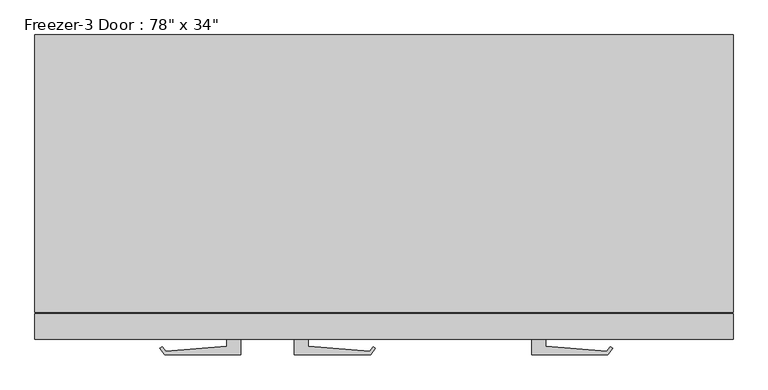
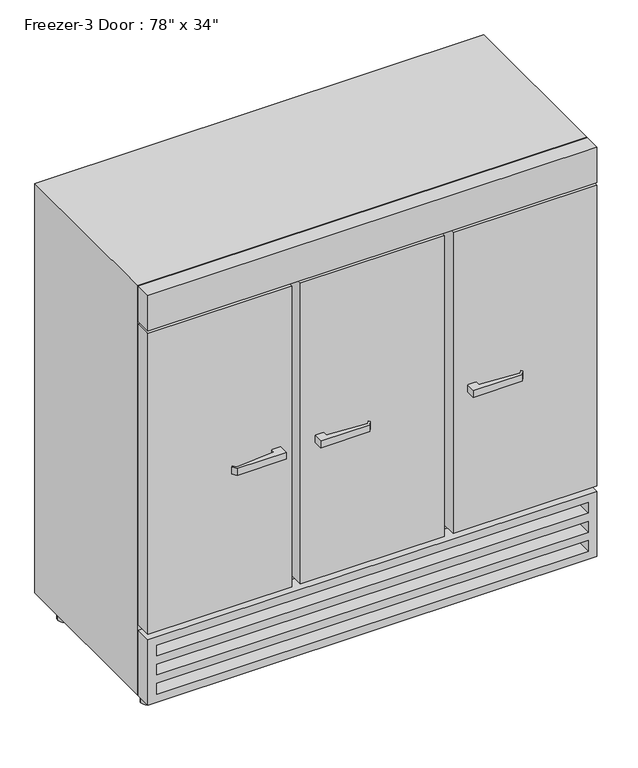
"""IFC4 building model written with IfcOpenShell, lengths in millimetres: proxy geometry."""

from ifc_helpers import new_model, si_unit, point, frame, frame_2d, origin, origin_with_axes, place, context, project, spatial, polyline, circle_curve, trimmed, segment, composite_curve, outline, extrude, source, transform, mapped, element, save


def proxy_233f0198(model_context):
    return source(origin(), model_context, "Body", "SweptSolid", [
        extrude(outline(polyline([(2012.95, 936.7988574), (2012.95, -1044.4011426), (101.6, -1044.4011426), (101.6, 936.7988574), (2012.95, 936.7988574)]), holes=[polyline([(1809.75, 911.3988574), (431.8, 911.3988574), (431.8, -1019.0011426), (1809.75, -1019.0011426), (1809.75, 911.3988574)])]), frame((0.0, -389.3849098, 0.0), z_axis=(0.0, 1.0, 0.0), x_axis=(0.0, 0.0, 1.0)), (0.0, 0.0, 1.0), 787.4),
        extrude(outline(polyline([(911.3988574, 372.6150902), (-1019.0011426, 372.6150902), (-1019.0011426, 398.0150902), (911.3988574, 398.0150902), (911.3988574, 372.6150902)])), frame((0.0, 0.0, 152.4), z_axis=(0.0, 0.0, 1.0), x_axis=(1.0, 0.0, 0.0)), (0.0, 0.0, 1.0), 1835.15),
        extrude(outline(polyline([(-409.4011426, -465.5849098), (-1044.4011426, -465.5849098), (-1044.4011426, -392.5599098), (-409.4011426, -392.5599098), (-409.4011426, -465.5849098)])), frame((0.0, 0.0, 431.8), z_axis=(0.0, 0.0, 1.0), x_axis=(1.0, 0.0, 0.0)), (0.0, 0.0, 1.0), 1403.35),
        extrude(outline(polyline([(936.7988574, -465.5849098), (-1044.4011426, -465.5849098), (-1044.4011426, -392.5599098), (936.7988574, -392.5599098), (936.7988574, -465.5849098)])), frame((0.0, 0.0, 1847.85), z_axis=(0.0, 0.0, 1.0), x_axis=(1.0, 0.0, 0.0)), (0.0, 0.0, 1.0), 165.1),
        extrude(outline(polyline([(406.4, 936.7988574), (406.4, -1044.4011426), (101.6, -1044.4011426), (101.6, 936.7988574), (406.4, 936.7988574)]), holes=[polyline([(368.3, 898.6988574), (317.5, 898.6988574), (317.5, -1006.3011426), (368.3, -1006.3011426), (368.3, 898.6988574)]), polyline([(279.4, 898.6988574), (228.6, 898.6988574), (228.6, -1006.3011426), (279.4, -1006.3011426), (279.4, 898.6988574)]), polyline([(190.5, 898.6988574), (139.7, 898.6988574), (139.7, -1006.3011426), (190.5, -1006.3011426), (190.5, 898.6988574)])]), frame((0.0, -465.5849098, 0.0), z_axis=(0.0, 1.0, 0.0), x_axis=(0.0, 0.0, 1.0)), (0.0, 0.0, 1.0), 73.025),
        extrude(outline(polyline([(936.7988574, -465.5849098), (301.9003887, -465.5849098), (301.9003887, -392.5599098), (936.7988574, -392.5599098), (936.7988574, -465.5849098)])), frame((0.0, 0.0, 431.8), z_axis=(0.0, 0.0, 1.0), x_axis=(1.0, 0.0, 0.0)), (0.0, 0.0, 1.0), 1403.35),
        extrude(outline(polyline([(263.8003887, -465.5849098), (-371.3011426, -465.5849098), (-371.3011426, -392.5599098), (263.8003887, -392.5599098), (263.8003887, -465.5849098)])), frame((0.0, 0.0, 431.8), z_axis=(0.0, 0.0, 1.0), x_axis=(1.0, 0.0, 0.0)), (0.0, 0.0, 1.0), 1403.35),
        extrude(outline(composite_curve([segment(trimmed(circle_curve(frame_2d((-961.8511426, 321.8150902)), 25.4), [point((-987.2511426, 321.8150902))], [point((-936.4511426, 321.8150902))], False, "CARTESIAN"), True, "CONTINUOUS"), segment(trimmed(circle_curve(frame_2d((-961.8511426, 321.8150902)), 25.4), [point((-936.4511426, 321.8150902))], [point((-987.2511426, 321.8150902))], False, "CARTESIAN"), True, "CONTINUOUS")], self_intersect=False)), origin_with_axes(), (0.0, 0.0, 1.0), 101.6),
        extrude(outline(composite_curve([segment(trimmed(circle_curve(frame_2d((854.2488574, 321.8150902)), 25.4), [point((828.8488574, 321.8150902))], [point((879.6488574, 321.8150902))], False, "CARTESIAN"), True, "CONTINUOUS"), segment(trimmed(circle_curve(frame_2d((854.2488574, 321.8150902)), 25.4), [point((879.6488574, 321.8150902))], [point((828.8488574, 321.8150902))], False, "CARTESIAN"), True, "CONTINUOUS")], self_intersect=False)), origin_with_axes(), (0.0, 0.0, 1.0), 101.6),
        extrude(outline(composite_curve([segment(trimmed(circle_curve(frame_2d((-961.8511426, -313.1849098)), 25.4), [point((-987.2511426, -313.1849098))], [point((-936.4511426, -313.1849098))], False, "CARTESIAN"), True, "CONTINUOUS"), segment(trimmed(circle_curve(frame_2d((-961.8511426, -313.1849098)), 25.4), [point((-936.4511426, -313.1849098))], [point((-987.2511426, -313.1849098))], False, "CARTESIAN"), True, "CONTINUOUS")], self_intersect=False)), origin_with_axes(), (0.0, 0.0, 1.0), 101.6),
        extrude(outline(composite_curve([segment(trimmed(circle_curve(frame_2d((854.2488574, -313.1849098)), 25.4), [point((828.8488574, -313.1849098))], [point((879.6488574, -313.1849098))], False, "CARTESIAN"), True, "CONTINUOUS"), segment(trimmed(circle_curve(frame_2d((854.2488574, -313.1849098)), 25.4), [point((879.6488574, -313.1849098))], [point((828.8488574, -313.1849098))], False, "CARTESIAN"), True, "CONTINUOUS")], self_intersect=False)), origin_with_axes(), (0.0, 0.0, 1.0), 101.6),
        extrude(outline(polyline([(-460.2011426, -509.9036861), (-676.1011426, -509.9036861), (-689.7759263, -491.3368406), (-683.2726974, -486.5471068), (-673.3243617, -500.0543926), (-499.3757581, -484.8358618), (-499.3757581, -465.5849098), (-460.2011426, -465.5849098), (-460.2011426, -509.9036861)])), frame((0.0, 0.0, 1071.927792), z_axis=(0.0, 0.0, 1.0), x_axis=(1.0, 0.0, 0.0)), (0.0, 0.0, 1.0), 31.75),
        extrude(outline(polyline([(-307.8011426, -509.9036861), (-307.8011426, -465.5849098), (-268.6265272, -465.5849098), (-268.6265272, -484.8358618), (-94.6779236, -500.0543926), (-84.7295879, -486.5471068), (-78.226359, -491.3368406), (-91.9011426, -509.9036861), (-307.8011426, -509.9036861)])), frame((0.0, 0.0, 1071.927792), z_axis=(0.0, 0.0, 1.0), x_axis=(1.0, 0.0, 0.0)), (0.0, 0.0, 1.0), 31.75),
        extrude(outline(polyline([(365.4003887, -509.9036861), (365.4003887, -465.5849098), (404.5750041, -465.5849098), (404.5750041, -484.8358618), (578.5236078, -500.0543926), (588.4719435, -486.5471068), (594.9751723, -491.3368406), (581.3003887, -509.9036861), (365.4003887, -509.9036861)])), frame((0.0, 0.0, 1071.927792), z_axis=(0.0, 0.0, 1.0), x_axis=(1.0, 0.0, 0.0)), (0.0, 0.0, 1.0), 31.75),
    ])


if __name__ == "__main__":
    model = new_model("IFC4")
    model_context = context("Model", 3, world=origin())
    ifc_project = project(units=[si_unit("LENGTHUNIT", "METRE", prefix="MILLI")], contexts=[model_context])
    site = spatial("IfcSite", under=ifc_project)
    building = spatial("IfcBuilding", under=site)
    placement = place(None, origin())
    proxy_shape = proxy_233f0198(model_context)
    element("IfcBuildingElementProxy", 1, Name="Freezer-3 Door : 78\" x 34\"", ObjectType="Freezer-3 Door : 78\" x 34\"", at=placement, inside=building, context=model_context, shape_type="MappedRepresentation", body=[
        mapped(proxy_shape, transform((0.0, 0.0, 0.0), x_axis=(1.0, 0.0, 0.0), y_axis=(0.0, 1.0, 0.0), z_axis=(0.0, 0.0, 1.0))),
    ])
    save(model, "model.ifc")

# Revit data of these elements
# Type "Freezer-3 Door : 78\" x 34\""
#   Assembly Code = "E1090320"
#   Description = "Reach-In Freezer"
#   Depth = 2' - 10"
#   Height = 6' - 7 1/4"
#   Width = 6' - 6"
#   Default Elevation = 0
# Element 1 (IfcBuildingElementProxy, "Freezer-3 Door : 78\" x 34\"")
#   Materials on its faces: "Metal - Stainless Steel", "Slate"
# Materials
#   "Metal - Stainless Steel": colour RGB 195 195 195, transparency 0
#   "Slate": colour RGB 127 127 127, transparency 0
